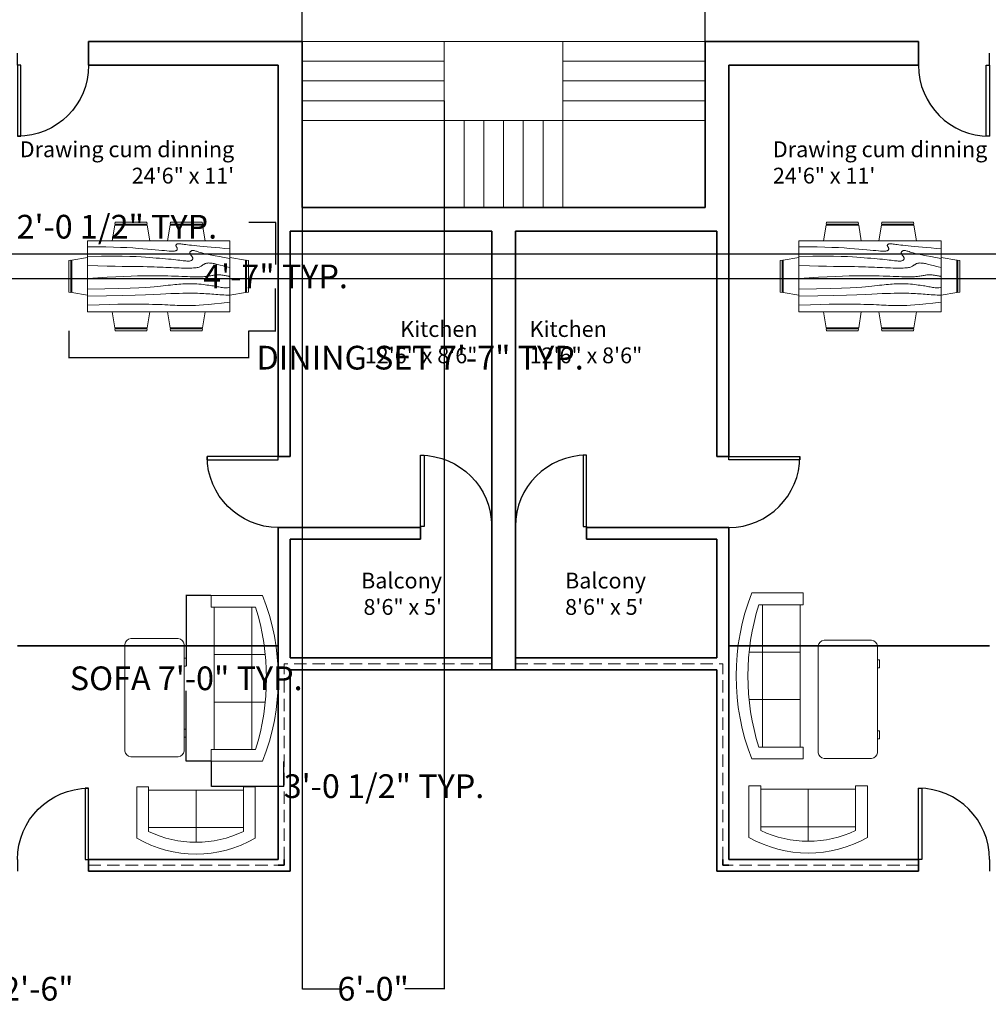
# Model space of a CAD drawing. Units: inches. Extents: x 2450 to 4494, y 1482 to 2597.
# Tile 5 of 7: x 3571 to 4062, y 1492 to 1990. Entities that reach past the tile are written whole.
import ezdxf

# ---------------------------------------------------------------- set-up
doc = ezdxf.new("R2010")
doc.units = ezdxf.units.IN
doc.header["$LTSCALE"] = 5
doc.header["$MEASUREMENT"] = 0
doc.linetypes.add('HIDDEN', pattern=[0.375, 0.25, -0.125])
for name, color, linetype, lineweight in [('A-ANNO-DIMS', 2, 'Continuous', 18), ('A-AREA-IDEN', 7, 'Continuous', 18), ('A-DOOR', 4, 'Continuous', 25), ('A-FLOR-STRS', 7, 'Continuous', 18), ('A-FURN', 8, 'Continuous', 18), ('A-WALL', 7, 'Continuous', 35), ('A-WALL-HIDN', 7, 'HIDDEN', 18)]:
    doc.layers.add(name, color=color, linetype=linetype, lineweight=lineweight)
doc.styles.get("Standard").update_dxf_attribs({"font": 'arial.ttf'})
doc.dimstyles.get("Standard").update_dxf_attribs({"dimtxt": 12, "dimasz": 0.18, "dimexe": 0.18, "dimexo": 0.0625, "dimgap": 0.09, "dimtad": 0, "dimtih": 1, "dimtoh": 1, "dimdec": 0, "dimzin": 0, "dimdsep": 46, "dimlunit": 3, "dimtxsty": 'Standard', "dimcen": 0.09, "dimadec": 0, "dimazin": 0, "dimtfac": 1, "dimtdec": 0, "dimtofl": 0, "dimtmove": 0, "dimatfit": 3, "dimfxl": 1, "dimtolj": 1, "dimtzin": 0, "dimarcsym": 0})

# ---------------------------------------------------------------- blocks, each defined once
blk = doc.blocks.new('*U4')
for p, q in [((-36, 0), (-36, -6)), ((0, 0), (0, -6))]:
    blk.add_line(p, q)
blk.add_lwpolyline([(0, 0), (0, 36), (-1.75, 36), (-1.75, 0)], close=True)
blk.add_arc((0, 0), 36, 90, 180)
blk = doc.blocks.new('*U2')
for p, q in [((0, 0), (0, -6)), ((36, 0), (36, -6))]:
    blk.add_line(p, q)
blk.add_lwpolyline([(0, 0), (0, 36), (1.75, 36), (1.75, 0)], close=True)
blk.add_arc((0, 0), 36, 0, 90)
blk = doc.blocks.new('*U5')
for p, q in [((-36, 0), (-36, 6)), ((0, 0), (0, 6))]:
    blk.add_line(p, q)
blk.add_lwpolyline([(0, 0), (0, -36), (-1.75, -36), (-1.75, 0)], close=True)
blk.add_arc((0, 0), 36, 180, 270)
blk = doc.blocks.new('Dining Set - 36 x 72 in.')
for p, q in [((-22.2343, 26.00059), (-23.4847, 17.99762)), ((-22.2304, 26), (-5.7608, 26)), ((-22, 27.5), (-22.1562, 26.50042)), ((-5.8416, 26.5), (-22.1534, 26.5)), ((-22, 27.5), (-6, 27.5)), ((-5.8437, 26.49966), (-6, 27.5)), ((-4.5152, 17.99762), (-5.7655, 25.99926)), ((5.7657, 26.00059), (4.5153, 17.99762)), ((5.7696, 26), (22.2392, 26)), ((6, 27.5), (5.8438, 26.50042)), ((22.1584, 26.5), (5.8466, 26.5)), ((6, 27.5), (22, 27.5)), ((22.1563, 26.49966), (22, 27.5)), ((23.4848, 17.99762), (22.2345, 25.99926)), ((36, 18), (-36, 18)), ((-36, 18), (-36, -18)), ((36, -18), (36, 18)), ((-45.5, 8), (-44.5004, 8.15617)), ((-45.5, 8), (-45.5, -8)), ((-44.5, -8.15843), (-44.5, 8.15338)), ((-44.0006, 8.23428), (-35.9976, 9.48474)), ((-44, 8.23041), (-44, -8.23915)), ((44.0006, 8.23428), (35.9976, 9.48474)), ((44, 8.23041), (44, -8.23915)), ((44.5, -8.15843), (44.5, 8.15338)), ((45.5, 8), (44.5005, 8.15617)), ((45.5, 8), (45.5, -8)), ((-44.4997, -8.15631), (-45.5, -8)), ((-35.9976, -9.48476), (-43.9993, -8.2345)), ((35.9976, -9.48476), (43.9993, -8.2345)), ((44.4997, -8.15631), (45.5, -8)), ((-36, -18), (36, -18)), ((-22.2343, -26.0006), (-23.4847, -17.99762)), ((-4.5152, -17.99762), (-5.7655, -25.99928)), ((5.7657, -26.0006), (4.5153, -17.99762)), ((23.4848, -17.99762), (22.2345, -25.99928)), ((-22.2304, -26), (-5.7608, -26)), ((-22, -27.5), (-22.1562, -26.50044)), ((-5.8416, -26.5), (-22.1534, -26.5)), ((-22, -27.5), (-6, -27.5)), ((-5.8437, -26.49967), (-6, -27.5)), ((5.7696, -26), (22.2392, -26)), ((6, -27.5), (5.8438, -26.50044)), ((22.1584, -26.5), (5.8466, -26.5)), ((6, -27.5), (22, -27.5)), ((22.1563, -26.49967), (22, -27.5))]:
    blk.add_line(p, q)
for points in [[(-36, 15), (-31.1772, 14.97754), (-26.8079, 14.91406), (-22.8538, 14.81543), (-19.276, 14.6875), (-16.0362, 14.53613), (-13.0957, 14.36718), (-10.4159, 14.18652), (-7.9583, 14), (-5.6904, 13.81315), (-3.6035, 13.63021), (-1.6954, 13.45508), (0.0365, 13.29166), (1.5945, 13.14388), (2.9811, 13.01562), (4.1988, 12.9108), (5.25, 12.83333), (6.1393, 12.78613), (6.8802, 12.76823), (7.4883, 12.77767), (7.9792, 12.8125), (8.3685, 12.87077), (8.6719, 12.95052), (8.9049, 13.0498), (9.0833, 13.16666), (9.2205, 13.29899), (9.3216, 13.44401), (9.3895, 13.59879), (9.4271, 13.76041), (9.4373, 13.92594), (9.4232, 14.09245), (9.3875, 14.257), (9.3333, 14.41666), (9.2638, 14.56917), (9.1836, 14.71484), (9.0975, 14.85465), (9.0104, 14.98958), (8.9272, 15.1206), (8.8529, 15.2487), (8.7922, 15.37483), (8.75, 15.5), (8.7305, 15.62467), (8.7344, 15.74739), (8.7617, 15.86621), (8.8125, 15.97916), (8.8867, 16.08431), (8.9844, 16.17968), (9.1055, 16.26334), (9.25, 16.33333), (9.4189, 16.38802), (9.6172, 16.42708), (9.8506, 16.45052), (10.125, 16.45833), (10.4463, 16.45052), (10.8203, 16.42708), (11.2529, 16.38802), (11.75, 16.33333), (12.3184, 16.26318), (12.9694, 16.17838), (13.7151, 16.07991), (14.5677, 15.96875), (15.5395, 15.84586), (16.6426, 15.71224), (17.8893, 15.56884), (19.2917, 15.41666), (20.859, 15.25667), (22.5879, 15.08984), (24.4721, 14.91715), (26.5052, 14.73958), (28.6809, 14.5581), (30.9929, 14.3737), (33.4347, 14.18733), (36, 14)], [(-36, 10), (-28.9766, 10.14274), (-23.1725, 10.20442), (-18.4241, 10.19775), (-14.5677, 10.13541), (-11.4399, 10.03011), (-8.877, 9.89453), (-6.7154, 9.74137), (-4.7917, 9.58333), (-2.9698, 9.43082), (-1.2246, 9.28515), (0.4415, 9.14534), (2.026, 9.01041), (3.5266, 8.87939), (4.9408, 8.7513), (6.266, 8.62516), (7.5, 8.5), (8.6411, 8.37549), (9.6914, 8.2539), (10.6538, 8.13818), (11.5312, 8.03125), (12.3267, 7.93603), (13.043, 7.85547), (13.6831, 7.79248), (14.25, 7.75), (14.7471, 7.7303), (15.1797, 7.73307), (15.5537, 7.75732), (15.875, 7.80208), (16.1494, 7.86637), (16.3828, 7.94922), (16.5811, 8.04964), (16.75, 8.16666), (16.8944, 8.29915), (17.0143, 8.44531), (17.1089, 8.60319), (17.1771, 8.77083), (17.218, 8.94629), (17.2305, 9.1276), (17.2137, 9.31282), (17.1667, 9.5), (17.0895, 9.6875), (16.987, 9.875), (16.8649, 10.0625), (16.7292, 10.25), (16.5856, 10.4375), (16.4401, 10.625), (16.2985, 10.8125), (16.1667, 11), (16.05, 11.18733), (15.9518, 11.3737), (15.8752, 11.5581), (15.8229, 11.73958), (15.798, 11.91715), (15.8034, 12.08984), (15.842, 12.25667), (15.9167, 12.41666), (16.0295, 12.56836), (16.1784, 12.70833), (16.3605, 12.83268), (16.5729, 12.9375), (16.8127, 13.01888), (17.0768, 13.07291), (17.3625, 13.0957), (17.6667, 13.08333), (17.9894, 13.03312), (18.3418, 12.94726), (18.7382, 12.82918), (19.1927, 12.68229), (19.7195, 12.51001), (20.3327, 12.31575), (21.0465, 12.10294), (21.875, 11.875), (22.8357, 11.63354), (23.959, 11.37304), (25.2786, 11.08618), (26.8282, 10.76562), (28.6414, 10.40405), (30.752, 9.99414), (33.1936, 9.52856), (36, 9)], [(-36, 5.5), (-30.7157, 5.3348), (-26.069, 5.20963), (-21.9946, 5.11767), (-18.4271, 5.05208), (-15.3009, 5.00602), (-12.5508, 4.97265), (-10.1112, 4.94515), (-7.9167, 4.91666), (-5.909, 4.88167), (-4.0586, 4.83984), (-2.3429, 4.79215), (-0.7396, 4.73958), (0.7739, 4.6831), (2.22, 4.6237), (3.6213, 4.56233), (5, 4.5), (6.373, 4.43782), (7.7344, 4.3776), (9.0723, 4.32129), (10.375, 4.27083), (11.6309, 4.22819), (12.8281, 4.19531), (13.9551, 4.17415), (15, 4.16666), (15.954, 4.17448), (16.819, 4.19791), (17.6001, 4.23698), (18.3021, 4.29166), (18.9299, 4.36198), (19.4883, 4.44791), (19.9823, 4.54948), (20.4167, 4.66666), (20.7969, 4.79899), (21.1302, 4.94401), (21.4245, 5.09879), (21.6875, 5.26041), (21.9271, 5.42594), (22.1511, 5.59245), (22.3672, 5.757), (22.5834, 5.91666), (22.8065, 6.06868), (23.0404, 6.21093), (23.2879, 6.34147), (23.5521, 6.45833), (23.8358, 6.55957), (24.142, 6.64323), (24.4735, 6.70735), (24.8334, 6.75), (25.2235, 6.76969), (25.642, 6.76692), (26.0858, 6.74267), (26.5521, 6.69791), (27.0379, 6.63362), (27.5404, 6.55078), (28.0565, 6.45036), (28.5834, 6.33333), (29.1242, 6.19987), (29.7071, 6.04687), (30.3661, 5.87044), (31.1354, 5.66666), (32.0493, 5.43164), (33.142, 5.16146), (34.4475, 4.85221), (36, 4.5)], [(-36, -1), (-30.7915, -0.6591), (-26.0195, -0.38216), (-21.6519, -0.16284), (-17.6563, 0.00521), (-14.0005, 0.12833), (-10.6523, 0.21289), (-7.5796, 0.26522), (-4.75, 0.29166), (-2.134, 0.29793), (0.2878, 0.28711), (2.5317, 0.26163), (4.6146, 0.22396), (6.5529, 0.17651), (8.3633, 0.12174), (10.0623, 0.06209), (11.6667, 0), (13.1899, -0.06201), (14.6341, -0.1211), (15.9982, -0.17432), (17.2813, -0.21875), (18.4823, -0.25147), (19.6003, -0.26953), (20.6343, -0.27002), (21.5834, -0.25), (22.4481, -0.20768), (23.2357, -0.14584), (23.9549, -0.06836), (24.6146, 0.02083), (25.2235, 0.11784), (25.7904, 0.21875), (26.3241, 0.31966), (26.8334, 0.41666), (27.3265, 0.50618), (27.8099, 0.58593), (28.2894, 0.65397), (28.7709, 0.70833), (29.2601, 0.74707), (29.763, 0.76823), (30.2855, 0.76985), (30.8334, 0.75), (31.4088, 0.70784), (31.9994, 0.64713), (32.589, 0.57275), (33.1615, 0.48958), (33.7008, 0.4025), (34.1908, 0.3164), (34.6153, 0.23616), (34.9584, 0.16666), (35.2099, 0.11165), (35.3848, 0.07031), (35.504, 0.04069), (35.5886, 0.02083), (35.6594, 0.00879), (35.7377, 0.0026), (35.8442, 0.00032), (36, 0)], [(-36, -6.5), (-27.1843, -6.31267), (-20.084, -6.1263), (-14.469, -5.9419), (-10.1094, -5.76042), (-6.7752, -5.58285), (-4.2363, -5.41016), (-2.2629, -5.24333), (-0.625, -5.08334), (0.8708, -4.93099), (2.2715, -4.78646), (3.5872, -4.64974), (4.8281, -4.52084), (6.0046, -4.39974), (7.127, -4.28646), (8.2053, -4.18099), (9.25, -4.08334), (10.2705, -3.99382), (11.2734, -3.91407), (12.2647, -3.84603), (13.25, -3.79167), (14.2354, -3.75293), (15.2266, -3.73177), (16.2295, -3.73015), (17.25, -3.75), (18.2912, -3.79248), (19.3451, -3.85547), (20.4009, -3.93604), (21.4479, -4.03125), (22.4754, -4.13819), (23.4727, -4.25391), (24.4289, -4.37549), (25.3334, -4.5), (26.1785, -4.62492), (26.9694, -4.74935), (27.7145, -4.87281), (28.4219, -4.99479), (29.1, -5.11483), (29.7572, -5.23242), (30.4016, -5.34709), (31.0417, -5.45834), (31.6837, -5.56437), (32.3262, -5.65821), (32.9658, -5.73153), (33.599, -5.77604), (34.2224, -5.78345), (34.8327, -5.74545), (35.4264, -5.65373), (36, -5.5)], [(-36, -10), (-26.4022, -9.81299), (-18.4675, -9.62891), (-11.9839, -9.45069), (-6.7396, -9.28125), (-2.5226, -9.12354), (0.8789, -8.98047), (3.6769, -8.85498), (6.0833, -8.75), (8.2767, -8.66765), (10.3021, -8.60677), (12.1712, -8.56543), (13.8958, -8.54167), (15.4876, -8.53353), (16.9583, -8.53907), (18.3197, -8.55632), (19.5834, -8.58334), (20.7616, -8.61841), (21.8685, -8.66081), (22.9188, -8.71004), (23.9271, -8.76563), (24.9081, -8.82707), (25.8763, -8.89388), (26.8465, -8.96558), (27.8334, -9.04167), (28.8474, -9.12118), (29.8828, -9.20117), (30.93, -9.27824), (31.9792, -9.34896), (33.0205, -9.40991), (34.0443, -9.45768), (35.0407, -9.48885), (36, -9.5)], [(-36, -14.5), (-30.0881, -14.33513), (-25.0332, -14.21224), (-20.7312, -14.12647), (-17.0781, -14.07292), (-13.97, -14.04671), (-11.3027, -14.04297), (-8.9724, -14.05681), (-6.875, -14.08334), (-4.9224, -14.11833), (-3.0905, -14.16016), (-1.3709, -14.20785), (0.2448, -14.26042), (1.7647, -14.3169), (3.1973, -14.3763), (4.5507, -14.43767), (5.8333, -14.5), (7.0554, -14.5621), (8.235, -14.62175), (9.3922, -14.67652), (10.5469, -14.72396), (11.7192, -14.76164), (12.929, -14.78711), (14.1965, -14.79794), (15.5417, -14.79167), (16.9933, -14.76424), (18.6152, -14.70508), (20.4804, -14.60197), (22.6615, -14.44271), (25.2312, -14.21509), (28.2624, -13.9069), (31.8277, -13.50594), (36, -13)]]:
    blk.add_lwpolyline(points)
blk = doc.blocks.new('Sofa - Roundback Loveseat 5 ft.')
for p, q in [((0, -32.44198), (0, -5.99998)), ((-24, -33.99998), (-24, -11.46958)), ((-23.9998, -13.38178), (23.99986, -13.38178)), ((24.00004, -33.99998), (24.00004, -11.46958)), ((-24, -32.44198), (24.00004, -32.44198))]:
    blk.add_line(p, q)
for points in [[(-24, -33.99998), (-30, -33.99998), (-30, -7.99998)], [(30.00004, -7.99998), (30.00004, -33.99998), (24.00004, -33.99998)]]:
    blk.add_lwpolyline(points)
for centre, radius, start, end in [((0, -60.24998), 60.24998, 60.13715, 119.8628), ((0, -61.38438), 55.38444, 64.32083, 115.6792)]:
    blk.add_arc(centre, radius, start, end)
blk = doc.blocks.new('Sofa - Roundback 7 ft.')
for p, q in [((-12.00002, -32.4421), (-12.00003, -6.5971)), ((11.99997, -32.4421), (11.99998, -6.5971)), ((-36.000027, -34), (-36.000027, -11.4696)), ((-35.999844, -13.3819), (35.9998, -13.3819)), ((35.99998, -34), (35.99998, -11.4696)), ((-36.000027, -32.4421), (35.99998, -32.4421))]:
    blk.add_line(p, q)
for points in [[(-36.000027, -34), (-42.000027, -34), (-42.000027, -8)], [(41.99998, -8), (41.99998, -34), (35.99998, -34)]]:
    blk.add_lwpolyline(points)
for centre, radius, start, end in [((0, -114.25), 114.25, 68.43141, 111.5686), ((-0.00001, -127.1968), 121.1968, 72.72033, 107.2797)]:
    blk.add_arc(centre, radius, start, end)
blk = doc.blocks.new('Desk - 30 x 60 in.')
for p, q in [((-26.999995, 0), (26.999995, 0)), ((-29.999995, -27), (-29.999995, -3)), ((29.999995, -3), (29.999995, -27)), ((26.999995, -30), (-26.999995, -30)), ((-20.000005, -30), (-20.000005, -31)), ((-20.000005, -31), (-16.000005, -31)), ((-16.000005, -31), (-16.000005, -30)), ((15.999995, -31), (15.999995, -30)), ((19.999995, -31), (15.999995, -31)), ((19.999995, -30), (19.999995, -31))]:
    blk.add_line(p, q)
for centre, start, end in [((-26.499995, -3.5), 98.1301, 171.8699), ((26.499995, -3.5), 8.130102, 81.8699), ((-26.499995, -26.5), 188.1301, 261.8699), ((26.499995, -26.5), 278.1301, 351.8699)]:
    blk.add_arc(centre, 3.535534, start, end)
blk = doc.blocks.new('*D55')
at = {"layer": 'A-ANNO-DIMS', "color": 0, "lineweight": -2, "ltscale": 5, "transparency": 16777216}
for p, q in [((3492.61, 1881.89), (3492.61, 1885.69)), ((3492.79, 1885.51), (3516.98, 1885.51)), ((3517.16, 1881.89), (3517.16, 1885.69)), ((3517.16, 1885.51), (3517.34, 1885.51))]:
    blk.add_line(p, q, dxfattribs=at)
at = {"layer": 'A-ANNO-DIMS', "color": 0, "ltscale": 5, "transparency": 16777216}
for points in [[(3492.79, 1885.54), (3492.79, 1885.48), (3492.61, 1885.51)], [(3516.98, 1885.54), (3516.98, 1885.48), (3517.16, 1885.51)]]:
    blk.add_solid(points, dxfattribs=at)
at = {"layer": 'Defpoints', "color": 0, "ltscale": 5, "transparency": 16777216}
for p in [(3517.16, 1885.51), (3492.61, 1881.83), (3517.16, 1881.83)]:
    blk.add_point(p, dxfattribs=at)
at = {"layer": 'A-ANNO-DIMS', "color": 0, "ltscale": 5, "transparency": 16777216, "insert": (3595.2, 1885.51), "char_height": 12, "attachment_point": 5}
blk.add_mtext('\\A1;BASIN 2\'-0 1/2" TYP.', dxfattribs=at)
blk = doc.blocks.new('*D59')
at = {"layer": 'A-ANNO-DIMS', "color": 0, "lineweight": -2, "ltscale": 5, "transparency": 16777216}
for p, q in [((3596.25, 1832.81), (3596.25, 1819.04)), ((3687.25, 1832.81), (3687.25, 1819.04)), ((3596.43, 1819.22), (3687.07, 1819.22)), ((3687.25, 1819.22), (3687.43, 1819.22))]:
    blk.add_line(p, q, dxfattribs=at)
at = {"layer": 'A-ANNO-DIMS', "color": 0, "ltscale": 5, "transparency": 16777216}
for points in [[(3596.43, 1819.25), (3596.43, 1819.19), (3596.25, 1819.22)], [(3687.07, 1819.25), (3687.07, 1819.19), (3687.25, 1819.22)]]:
    blk.add_solid(points, dxfattribs=at)
at = {"layer": 'Defpoints', "color": 0, "ltscale": 5, "transparency": 16777216}
for p in [(3596.25, 1832.87), (3687.25, 1832.87), (3687.25, 1819.22)]:
    blk.add_point(p, dxfattribs=at)
at = {"layer": 'A-ANNO-DIMS', "color": 0, "ltscale": 5, "transparency": 16777216, "insert": (3774.09, 1819.22), "char_height": 12, "attachment_point": 5}
blk.add_mtext('\\A1;DINING SET 7\'-7" TYP.', dxfattribs=at)
blk = doc.blocks.new('*D60')
at = {"layer": 'A-ANNO-DIMS', "color": 0, "lineweight": -2, "ltscale": 5, "transparency": 16777216}
for p, q in [((3687.31, 1887.87), (3701.08, 1887.87)), ((3700.9, 1887.69), (3700.9, 1866.46)), ((3700.9, 1833.05), (3700.9, 1854.28)), ((3687.31, 1832.87), (3701.08, 1832.87))]:
    blk.add_line(p, q, dxfattribs=at)
at = {"layer": 'A-ANNO-DIMS', "color": 0, "ltscale": 5, "transparency": 16777216}
for points in [[(3700.87, 1887.69), (3700.93, 1887.69), (3700.9, 1887.87)], [(3700.87, 1833.05), (3700.93, 1833.05), (3700.9, 1832.87)]]:
    blk.add_solid(points, dxfattribs=at)
at = {"layer": 'Defpoints', "color": 0, "ltscale": 5, "transparency": 16777216}
for p in [(3687.25, 1887.87), (3700.9, 1887.87), (3687.25, 1832.87)]:
    blk.add_point(p, dxfattribs=at)
at = {"layer": 'A-ANNO-DIMS', "color": 0, "ltscale": 5, "transparency": 16777216, "insert": (3700.9, 1860.37), "char_height": 12, "attachment_point": 5}
blk.add_mtext('\\A1;4\'-7" TYP.', dxfattribs=at)
blk = doc.blocks.new('*D63')
at = {"layer": 'A-ANNO-DIMS', "color": 0, "lineweight": -2, "ltscale": 5, "transparency": 16777216}
for p, q in [((3668.23, 1698.91), (3655.51, 1698.91)), ((3655.69, 1698.73), (3655.69, 1663.2)), ((3655.69, 1615.09), (3655.69, 1650.61)), ((3668.23, 1614.91), (3655.51, 1614.91))]:
    blk.add_line(p, q, dxfattribs=at)
at = {"layer": 'A-ANNO-DIMS', "color": 0, "ltscale": 5, "transparency": 16777216}
for points in [[(3655.66, 1698.73), (3655.72, 1698.73), (3655.69, 1698.91)], [(3655.66, 1615.09), (3655.72, 1615.09), (3655.69, 1614.91)]]:
    blk.add_solid(points, dxfattribs=at)
at = {"layer": 'Defpoints', "color": 0, "ltscale": 5, "transparency": 16777216}
for p in [(3668.29, 1698.91), (3655.69, 1614.91), (3668.29, 1614.91)]:
    blk.add_point(p, dxfattribs=at)
at = {"layer": 'A-ANNO-DIMS', "color": 0, "ltscale": 5, "transparency": 16777216, "insert": (3655.69, 1656.91), "char_height": 12, "attachment_point": 5}
blk.add_mtext('\\A1;SOFA 7\'-0" TYP.', dxfattribs=at)
blk = doc.blocks.new('*D64')
at = {"layer": 'A-ANNO-DIMS', "color": 0, "lineweight": -2, "ltscale": 5, "transparency": 16777216}
for p, q in [((3668.29, 1614.84), (3668.29, 1602.13)), ((3704.96, 1614.84), (3704.96, 1602.13)), ((3668.47, 1602.31), (3704.78, 1602.31)), ((3704.96, 1602.31), (3705.14, 1602.31))]:
    blk.add_line(p, q, dxfattribs=at)
at = {"layer": 'A-ANNO-DIMS', "color": 0, "ltscale": 5, "transparency": 16777216}
for points in [[(3668.47, 1602.34), (3668.47, 1602.28), (3668.29, 1602.31)], [(3704.78, 1602.34), (3704.78, 1602.28), (3704.96, 1602.31)]]:
    blk.add_solid(points, dxfattribs=at)
at = {"layer": 'Defpoints', "color": 0, "ltscale": 5, "transparency": 16777216}
for p in [(3668.29, 1614.91), (3704.96, 1614.91), (3704.96, 1602.31)]:
    blk.add_point(p, dxfattribs=at)
at = {"layer": 'A-ANNO-DIMS', "color": 0, "ltscale": 5, "transparency": 16777216, "insert": (3755.78, 1602.31), "char_height": 12, "attachment_point": 5}
blk.add_mtext('\\A1;3\'-0 1/2" TYP.', dxfattribs=at)
blk = doc.blocks.new('*D73')
at = {"layer": 'A-ANNO-DIMS', "color": 0, "lineweight": -2, "ltscale": 5, "transparency": 16777216}
for p, q in [((3714.29, 1979.33), (3714.29, 2578.95)), ((3714.47, 2578.77), (3796.15, 2578.77)), ((3918.11, 2578.77), (3836.43, 2578.77)), ((3918.29, 1979.33), (3918.29, 2578.95))]:
    blk.add_line(p, q, dxfattribs=at)
at = {"layer": 'A-ANNO-DIMS', "color": 0, "ltscale": 5, "transparency": 16777216}
for points in [[(3714.47, 2578.8), (3714.47, 2578.74), (3714.29, 2578.77)], [(3918.11, 2578.8), (3918.11, 2578.74), (3918.29, 2578.77)]]:
    blk.add_solid(points, dxfattribs=at)
at = {"layer": 'Defpoints', "color": 0, "ltscale": 5, "transparency": 16777216}
for p in [(3918.29, 2578.77), (3714.29, 1979.27), (3918.29, 1979.27)]:
    blk.add_point(p, dxfattribs=at)
at = {"layer": 'A-ANNO-DIMS', "color": 0, "ltscale": 5, "transparency": 16777216, "insert": (3816.29, 2578.77), "char_height": 12, "attachment_point": 5}
blk.add_mtext('\\A1;17\'-0"', dxfattribs=at)
blk = doc.blocks.new('*D74')
at = {"layer": 'A-ANNO-DIMS', "color": 0, "lineweight": -2, "ltscale": 5, "transparency": 16777216}
for p, q in [((3786.29, 1949.2), (3786.29, 1499.59)), ((3714.29, 1939.2), (3714.29, 1499.59)), ((3714.47, 1499.77), (3734.22, 1499.77)), ((3786.11, 1499.77), (3766.36, 1499.77))]:
    blk.add_line(p, q, dxfattribs=at)
at = {"layer": 'A-ANNO-DIMS', "color": 0, "ltscale": 5, "transparency": 16777216}
for points in [[(3714.47, 1499.8), (3714.47, 1499.74), (3714.29, 1499.77)], [(3786.11, 1499.8), (3786.11, 1499.74), (3786.29, 1499.77)]]:
    blk.add_solid(points, dxfattribs=at)
at = {"layer": 'Defpoints', "color": 0, "ltscale": 5, "transparency": 16777216}
for p in [(3786.29, 1949.27), (3714.29, 1939.27), (3786.29, 1499.77)]:
    blk.add_point(p, dxfattribs=at)
at = {"layer": 'A-ANNO-DIMS', "color": 0, "ltscale": 5, "transparency": 16777216, "insert": (3750.29, 1499.77), "char_height": 12, "attachment_point": 5}
blk.add_mtext('\\A1;6\'-0"', dxfattribs=at)
blk = doc.blocks.new('*D83')
at = {"layer": 'A-ANNO-DIMS', "color": 0, "lineweight": -2, "ltscale": 5, "transparency": 16777216}
for p, q in [((3534.29, 1859.2), (3534.29, 1499.59)), ((3564.29, 1859.2), (3564.29, 1499.59)), ((3534.47, 1499.77), (3564.11, 1499.77)), ((3564.29, 1499.77), (3564.47, 1499.77))]:
    blk.add_line(p, q, dxfattribs=at)
at = {"layer": 'A-ANNO-DIMS', "color": 0, "ltscale": 5, "transparency": 16777216}
for points in [[(3534.47, 1499.8), (3534.47, 1499.74), (3534.29, 1499.77)], [(3564.11, 1499.8), (3564.11, 1499.74), (3564.29, 1499.77)]]:
    blk.add_solid(points, dxfattribs=at)
at = {"layer": 'Defpoints', "color": 0, "ltscale": 5, "transparency": 16777216}
for p in [(3534.29, 1859.27), (3564.29, 1859.27), (3564.29, 1499.77)]:
    blk.add_point(p, dxfattribs=at)
at = {"layer": 'A-ANNO-DIMS', "color": 0, "ltscale": 5, "transparency": 16777216, "insert": (3580.61, 1499.77), "char_height": 12, "attachment_point": 5}
blk.add_mtext('\\A1;2\'-6"', dxfattribs=at)
blk = doc.blocks.new('*D87')
at = {"layer": 'A-ANNO-DIMS', "color": 0, "lineweight": -2, "ltscale": 5, "transparency": 16777216}
for p, q in [((3504.95, 1871.76), (4433.97, 1871.76)), ((4433.79, 1871.76), (4433.79, 1871.94)), ((4433.79, 1871.94), (4433.97, 1871.94)), ((4433.79, 1859.45), (4433.79, 1871.58)), ((3534.35, 1859.27), (4433.97, 1859.27))]:
    blk.add_line(p, q, dxfattribs=at)
at = {"layer": 'A-ANNO-DIMS', "color": 0, "ltscale": 5, "transparency": 16777216}
for points in [[(4433.76, 1871.58), (4433.82, 1871.58), (4433.79, 1871.76)], [(4433.76, 1859.45), (4433.82, 1859.45), (4433.79, 1859.27)]]:
    blk.add_solid(points, dxfattribs=at)
at = {"layer": 'Defpoints', "color": 0, "ltscale": 5, "transparency": 16777216}
for p in [(3504.89, 1871.76), (4433.79, 1871.76), (3534.29, 1859.27)]:
    blk.add_point(p, dxfattribs=at)
at = {"layer": 'A-ANNO-DIMS', "color": 0, "ltscale": 5, "transparency": 16777216, "insert": (4463.43, 1871.94), "char_height": 12, "attachment_point": 5}
blk.add_mtext('\\A1;1\'-0 1/2"', dxfattribs=at)

msp = doc.modelspace()

# ---------------------------------------------------------------- linework, layer by layer
at = {"layer": 'A-FLOR-STRS', "ltscale": 5}
for p, q in [((3714.29, 1979.27), (3918.29, 1979.27)), ((3714.29, 1969.27), (3786.29, 1969.27)), ((3846.29, 1969.27), (3918.29, 1969.27)), ((3714.29, 1959.27), (3786.29, 1959.27)), ((3846.29, 1959.27), (3918.29, 1959.27)), ((3714.29, 1949.27), (3786.29, 1949.27)), ((3846.29, 1949.27), (3918.29, 1949.27)), ((3714.29, 1939.27), (3918.29, 1939.27)), ((3796.29, 1939.27), (3796.29, 1895.27)), ((3806.29, 1939.27), (3806.29, 1895.27)), ((3816.29, 1939.27), (3816.29, 1895.27)), ((3826.29, 1939.27), (3826.29, 1895.27)), ((3836.29, 1939.27), (3836.29, 1895.27)), ((3846.29, 1939.27), (3846.29, 1895.27))]:
    msp.add_line(p, q, dxfattribs=at)
at = {"layer": 'A-FLOR-STRS'}
for p, q in [((3786.29, 1979.27), (3786.29, 1895.27)), ((3846.29, 1979.27), (3846.29, 1895.27))]:
    msp.add_line(p, q, dxfattribs=at)
at = {"layer": 'A-WALL'}
for p, q in [((3606.29, 1979.27), (3714.29, 1979.27)), ((3606.29, 1967.27), (3606.29, 1979.27)), ((3714.29, 1967.27), (3714.29, 1979.27)), ((4026.29, 1979.27), (3918.29, 1979.27)), ((3918.29, 1967.27), (3918.29, 1979.27)), ((4026.29, 1967.27), (4026.29, 1979.27)), ((3606.29, 1967.27), (3702.29, 1967.27)), ((3702.29, 1967.27), (3702.29, 1769.27)), ((3714.29, 1967.27), (3714.29, 1895.27)), ((3918.29, 1967.27), (3918.29, 1895.27)), ((4026.29, 1967.27), (3930.29, 1967.27)), ((3930.29, 1967.27), (3930.29, 1769.27)), ((3714.29, 1895.27), (3810.29, 1895.27)), ((3822.29, 1895.27), (3810.29, 1895.27)), ((3810.29, 1895.27), (3822.29, 1895.27)), ((3918.29, 1895.27), (3822.29, 1895.27)), ((3708.29, 1883.27), (3810.29, 1883.27)), ((3708.29, 1883.27), (3708.29, 1769.27)), ((3810.29, 1883.27), (3810.29, 1733.27)), ((3822.29, 1883.27), (3822.29, 1661.27)), ((3924.29, 1883.27), (3822.29, 1883.27)), ((3822.29, 1883.27), (3822.29, 1733.27)), ((3822.29, 1883.27), (3822.29, 1661.27)), ((3924.29, 1883.27), (3924.29, 1769.27)), ((3708.29, 1769.27), (3702.29, 1769.27)), ((3924.29, 1769.27), (3930.29, 1769.27)), ((3702.29, 1733.27), (3702.29, 1565.27)), ((3708.29, 1733.27), (3702.29, 1733.27)), ((3708.29, 1733.27), (3774.29, 1733.27)), ((3774.29, 1733.27), (3774.29, 1727.27)), ((3810.29, 1733.27), (3810.29, 1727.27)), ((3822.29, 1733.27), (3822.29, 1727.27)), ((3924.29, 1733.27), (3858.29, 1733.27)), ((3858.29, 1733.27), (3858.29, 1727.27)), ((3924.29, 1733.27), (3930.29, 1733.27)), ((3930.29, 1733.27), (3930.29, 1565.27)), ((3708.29, 1727.27), (3774.29, 1727.27)), ((3708.29, 1727.27), (3708.29, 1667.27)), ((3810.29, 1727.27), (3810.29, 1667.27)), ((3822.29, 1727.27), (3822.29, 1667.27)), ((3924.29, 1727.27), (3858.29, 1727.27)), ((3924.29, 1727.27), (3924.29, 1667.27)), ((3570.29, 1673.27), (3702.29, 1673.27)), ((4062.29, 1673.27), (3930.29, 1673.27)), ((3708.29, 1667.27), (3810.29, 1667.27)), ((3810.29, 1667.27), (3810.29, 1661.27)), ((3924.29, 1667.27), (3822.29, 1667.27)), ((3822.29, 1667.27), (3822.29, 1661.27)), ((3708.29, 1661.27), (3810.29, 1661.27)), ((3708.29, 1661.27), (3708.29, 1571.27)), ((3822.29, 1661.27), (3810.29, 1661.27)), ((3810.29, 1661.27), (3822.29, 1661.27)), ((3924.29, 1661.27), (3822.29, 1661.27)), ((3924.29, 1661.27), (3924.29, 1571.27)), ((3708.29, 1571.27), (3708.29, 1559.27)), ((3924.29, 1571.27), (3924.29, 1559.27)), ((3702.29, 1565.27), (3606.29, 1565.27)), ((3606.29, 1565.27), (3606.29, 1559.27)), ((3705.29, 1565.27), (3705.29, 1562.27)), ((3927.29, 1565.27), (3927.29, 1562.27)), ((3930.29, 1565.27), (4026.29, 1565.27)), ((4026.29, 1565.27), (4026.29, 1559.27)), ((3702.29, 1562.27), (3705.29, 1562.27)), ((3930.29, 1562.27), (3927.29, 1562.27)), ((3708.29, 1559.27), (3606.29, 1559.27)), ((3924.29, 1559.27), (4026.29, 1559.27))]:
    msp.add_line(p, q, dxfattribs=at)
at = {"layer": 'A-WALL-HIDN', "ltscale": 5}
for p, q in [((3705.29, 1565.27), (3705.29, 1664.27)), ((3810.29, 1664.27), (3705.34, 1664.27)), ((3822.29, 1664.27), (3927.24, 1664.27)), ((3927.29, 1565.27), (3927.29, 1664.27)), ((3606.29, 1562.27), (3702.29, 1562.27)), ((4026.29, 1562.27), (3930.29, 1562.27))]:
    msp.add_line(p, q, dxfattribs=at)

# ---------------------------------------------------------------- block references
at = {"layer": 'A-DOOR', "xscale": -1}
for name, p in [('*U5', (3570.29, 1967.27)), ('*U4', (3774.29, 1733.8)), ('*U2', (3606.29, 1565.27))]:
    msp.add_blockref(name, p, dxfattribs=at)
at = {"layer": 'A-DOOR'}
for name, p in [('*U5', (4062.29, 1967.27)), ('*U4', (3858.29, 1733.8)), ('*U2', (4026.29, 1565.27))]:
    msp.add_blockref(name, p, dxfattribs=at)
at = {"layer": 'A-DOOR', "xscale": -1, "rotation": 90}
msp.add_blockref('*U2', (3702.29, 1769.27), dxfattribs=at)
at = {"layer": 'A-DOOR', "rotation": 270}
msp.add_blockref('*U2', (3930.29, 1769.27), dxfattribs=at)
at = {"layer": 'A-FURN', "ltscale": 5}
for p in [(3641.75, 1860.37), (4001.8, 1860.37)]:
    msp.add_blockref('Dining Set - 36 x 72 in.', p, dxfattribs=at)
for name, p, rotation in [('Sofa - Roundback 7 ft.', (3934, 1658.1), 90), ('Sofa - Roundback 7 ft.', (3702.29, 1656.91), 270), ('Desk - 30 x 60 in.', (3624.64, 1647.1), 90), ('Desk - 30 x 60 in.', (3975.55, 1646.27), 90), ('Sofa - Roundback Loveseat 5 ft.', (3660.64, 1567.93), 180), ('Sofa - Roundback Loveseat 5 ft.', (3970.5, 1568.41), 180)]:
    msp.add_blockref(name, p, dxfattribs=dict(at, rotation=rotation))

# ---------------------------------------------------------------- texts
at = {"layer": 'A-AREA-IDEN', "char_height": 8}
for s, insert, attachment_point in [('Drawing cum dinning\\P24\'6" x 11\'', (3679.96, 1928.7), 3), ('Drawing cum dinning\\P24\'6" x 11\'', (3952.62, 1928.7), 1), ('Kitchen\\P12\'6" x 8\'6"', (3803.09, 1837.72), 3), ('Kitchen\\P12\'6" x 8\'6"', (3829.49, 1837.72), 1), ('Balcony\\P8\'6" x 5\'', (3785.14, 1710.38), 3), ('Balcony\\P8\'6" x 5\'', (3847.44, 1710.38), 1)]:
    msp.add_mtext_dynamic_manual_height_columns(s, width=155.5618, gutter_width=1, heights=[0], dxfattribs=dict(at, insert=insert, attachment_point=attachment_point))

# ---------------------------------------------------------------- dimensions: what is measured, and where the dimension line sits
at = {"layer": 'A-ANNO-DIMS', "ltscale": 5}
for base, p1, p2, picture, middle in [((3918.29, 2578.77), (3714.29, 1979.27), (3918.29, 1979.27), '*D73', (3816.29, 2578.77)), ((3786.29, 1499.77), (3714.29, 1939.27), (3786.29, 1949.27), '*D74', (3750.29, 1499.77)), ((3564.29, 1499.77), (3534.29, 1859.27), (3564.29, 1859.27), '*D83', (3580.61, 1499.77))]:
    dim = msp.add_linear_dim(base=base, p1=p1, p2=p2, dimstyle='Standard', override={"dimdec": 1, "dimlfac": 1, "dimrnd": 0, "dimzin": 1, "dimdsep": 46, "dimlunit": 4, "dimfrac": 2}, dxfattribs=at)
    dim.commit()
    dim.dimension.update_dxf_attribs({"geometry": picture, "text_midpoint": middle})
for base, p1, p2, text, picture, middle in [((3517.1616, 1885.5149), (3492.6107, 1881.8322), (3517.1616, 1881.8322), 'BASIN <> TYP.', '*D55', (3595.2024, 1885.5149)), ((3687.25, 1819.22), (3596.25, 1832.87), (3687.25, 1832.87), 'DINING SET <> TYP.', '*D59', (3774.09, 1819.22)), ((3704.96, 1602.31), (3668.29, 1614.91), (3704.96, 1614.91), '<> TYP.', '*D64', (3755.78, 1602.31))]:
    dim = msp.add_linear_dim(base=base, p1=p1, p2=p2, text=text, dimstyle='Standard', override={"dimdec": 1, "dimlfac": 1, "dimrnd": 0, "dimzin": 1, "dimdsep": 46, "dimlunit": 4, "dimfrac": 2}, dxfattribs=at)
    dim.commit()
    dim.dimension.update_dxf_attribs({"geometry": picture, "text_midpoint": middle})
dim = msp.add_linear_dim(base=(4433.79, 1871.76), p1=(3534.29, 1859.27), p2=(3504.89, 1871.76), angle=90, dimstyle='Standard', override={"dimdec": 1, "dimlfac": 1, "dimrnd": 0, "dimzin": 1, "dimdsep": 46, "dimlunit": 4, "dimfrac": 2}, dxfattribs=at)
dim.commit()
dim.dimension.update_dxf_attribs({"geometry": '*D87', "text_midpoint": (4463.43, 1871.94)})
for base, p1, p2, angle, text, picture, middle in [((3700.9, 1887.87), (3687.25, 1832.87), (3687.25, 1887.87), 90, '<> TYP.', '*D60', (3700.9, 1860.37)), ((3655.69, 1614.91), (3668.29, 1698.91), (3668.29, 1614.91), 270, 'SOFA <> TYP.', '*D63', (3655.69, 1656.91))]:
    dim = msp.add_linear_dim(base=base, p1=p1, p2=p2, angle=angle, text=text, dimstyle='Standard', override={"dimdec": 1, "dimlfac": 1, "dimrnd": 0, "dimzin": 1, "dimdsep": 46, "dimlunit": 4, "dimfrac": 2}, dxfattribs=at)
    dim.commit()
    dim.dimension.update_dxf_attribs({"geometry": picture, "text_midpoint": middle})

doc.saveas('drawing.dxf')
